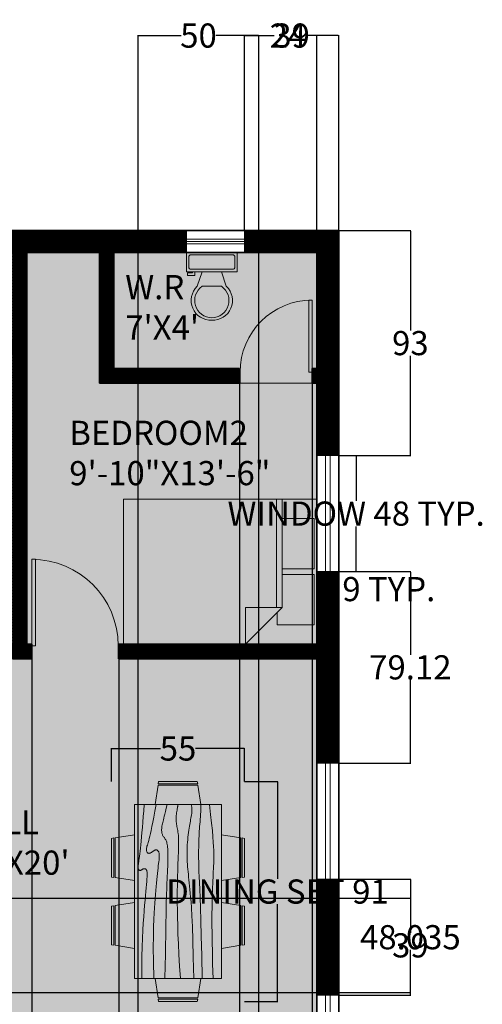
# Model space of a CAD drawing. Units: inches. Extents: x -89252 to 1164, y -183799 to 823.
# Tile 4 of 4: x 972 to 1164, y 416 to 823. Entities that reach past the tile are written whole.
import ezdxf

# ---------------------------------------------------------------- set-up
doc = ezdxf.new("R2010")
doc.units = ezdxf.units.IN
doc.header["$MEASUREMENT"] = 0
for name, color, linetype, lineweight in [('A-ANNO-DIMS', 2, 'Continuous', 18), ('A-AREA-IDEN', 7, 'Continuous', 25), ('A-FURN', 8, 'Continuous', 18), ('A-GLAZ', 4, 'Continuous', 18), ('A-WALL', 7, 'Continuous', 35), ('BED', 7, 'Continuous', 18), ('DOOR', 7, 'Continuous', 18), ('TOILET', 7, 'Continuous', 18)]:
    doc.layers.add(name, color=color, linetype=linetype, lineweight=lineweight)
doc.layers.add('A-FLOR-PATT', color=252, linetype='Continuous', lineweight=13, true_color=0x939598)
doc.layers.add('A-WALL-PATT', color=18, linetype='Continuous', lineweight=13, true_color=0x000000)
doc.styles.get("Standard").update_dxf_attribs({"font": 'arial.ttf'})
doc.dimstyles.get("Standard").update_dxf_attribs({"dimtxt": 10, "dimasz": 0.18, "dimexe": 0.18, "dimexo": 0.0625, "dimgap": 0.09, "dimtad": 0, "dimtih": 1, "dimtoh": 1, "dimdec": 0, "dimzin": 0, "dimdsep": 46, "dimlunit": 3, "dimtxsty": 'Standard', "dimcen": 0.09, "dimadec": 0, "dimazin": 0, "dimtfac": 1, "dimtdec": 0, "dimtofl": 0, "dimtmove": 0, "dimatfit": 3, "dimfxl": 1, "dimtolj": 1, "dimtzin": 0, "dimarcsym": 0})

# ---------------------------------------------------------------- blocks, each defined once
blk = doc.blocks.new('*U3')
for p, q in [((0, 0), (0, -6)), ((40, 0), (40, -6))]:
    blk.add_line(p, q)
blk.add_lwpolyline([(0, 0), (0, 40), (1.75, 40), (1.75, 0)], close=True)
blk.add_arc((0, 0), 40, 0, 90)
blk = doc.blocks.new('Dining Set - 36 x 72 in.')
for p, q in [((-22.2343, 26.00059), (-23.4847, 17.99762)), ((-22.2304, 26), (-5.7608, 26)), ((-22, 27.5), (-22.1562, 26.50042)), ((-5.8416, 26.5), (-22.1534, 26.5)), ((-22, 27.5), (-6, 27.5)), ((-5.8437, 26.49966), (-6, 27.5)), ((-4.5152, 17.99762), (-5.7655, 25.99926)), ((5.7657, 26.00059), (4.5153, 17.99762)), ((5.7696, 26), (22.2392, 26)), ((6, 27.5), (5.8438, 26.50042)), ((22.1584, 26.5), (5.8466, 26.5)), ((6, 27.5), (22, 27.5)), ((22.1563, 26.49966), (22, 27.5)), ((23.4848, 17.99762), (22.2345, 25.99926)), ((36, 18), (-36, 18)), ((-36, 18), (-36, -18)), ((36, -18), (36, 18)), ((-45.5, 8), (-44.5004, 8.15617)), ((-44.5, -8.15843), (-44.5, 8.15338)), ((-44.0006, 8.23428), (-35.9976, 9.48474)), ((-44, 8.23041), (-44, -8.23915)), ((44.0006, 8.23428), (35.9976, 9.48474)), ((44, 8.23041), (44, -8.23915)), ((44.5, -8.15843), (44.5, 8.15338)), ((45.5, 8), (44.5005, 8.15617)), ((-45.5, 8), (-45.5, -8)), ((45.5, 8), (45.5, -8)), ((-44.4997, -8.15631), (-45.5, -8)), ((44.4997, -8.15631), (45.5, -8)), ((-35.9976, -9.48476), (-43.9993, -8.2345)), ((35.9976, -9.48476), (43.9993, -8.2345)), ((-36, -18), (36, -18)), ((-22.2343, -26.0006), (-23.4847, -17.99762)), ((-4.5152, -17.99762), (-5.7655, -25.99928)), ((5.7657, -26.0006), (4.5153, -17.99762)), ((23.4848, -17.99762), (22.2345, -25.99928)), ((-22.2304, -26), (-5.7608, -26)), ((-22, -27.5), (-22.1562, -26.50044)), ((-5.8416, -26.5), (-22.1534, -26.5)), ((-22, -27.5), (-6, -27.5)), ((-5.8437, -26.49967), (-6, -27.5)), ((5.7696, -26), (22.2392, -26)), ((6, -27.5), (5.8438, -26.50044)), ((22.1584, -26.5), (5.8466, -26.5)), ((6, -27.5), (22, -27.5)), ((22.1563, -26.49967), (22, -27.5))]:
    blk.add_line(p, q)
for points in [[(-36, 15), (-31.1772, 14.97754), (-26.8079, 14.91406), (-22.8538, 14.81543), (-19.276, 14.6875), (-16.0362, 14.53613), (-13.0957, 14.36718), (-10.4159, 14.18652), (-7.9583, 14), (-5.6904, 13.81315), (-3.6035, 13.63021), (-1.6954, 13.45508), (0.0365, 13.29166), (1.5945, 13.14388), (2.9811, 13.01562), (4.1988, 12.9108), (5.25, 12.83333), (6.1393, 12.78613), (6.8802, 12.76823), (7.4883, 12.77767), (7.9792, 12.8125), (8.3685, 12.87077), (8.6719, 12.95052), (8.9049, 13.0498), (9.0833, 13.16666), (9.2205, 13.29899), (9.3216, 13.44401), (9.3895, 13.59879), (9.4271, 13.76041), (9.4373, 13.92594), (9.4232, 14.09245), (9.3875, 14.257), (9.3333, 14.41666), (9.2638, 14.56917), (9.1836, 14.71484), (9.0975, 14.85465), (9.0104, 14.98958), (8.9272, 15.1206), (8.8529, 15.2487), (8.7922, 15.37483), (8.75, 15.5), (8.7305, 15.62467), (8.7344, 15.74739), (8.7617, 15.86621), (8.8125, 15.97916), (8.8867, 16.08431), (8.9844, 16.17968), (9.1055, 16.26334), (9.25, 16.33333), (9.4189, 16.38802), (9.6172, 16.42708), (9.8506, 16.45052), (10.125, 16.45833), (10.4463, 16.45052), (10.8203, 16.42708), (11.2529, 16.38802), (11.75, 16.33333), (12.3184, 16.26318), (12.9694, 16.17838), (13.7151, 16.07991), (14.5677, 15.96875), (15.5395, 15.84586), (16.6426, 15.71224), (17.8893, 15.56884), (19.2917, 15.41666), (20.859, 15.25667), (22.5879, 15.08984), (24.4721, 14.91715), (26.5052, 14.73958), (28.6809, 14.5581), (30.9929, 14.3737), (33.4347, 14.18733), (36, 14)], [(-36, 10), (-28.9766, 10.14274), (-23.1725, 10.20442), (-18.4241, 10.19775), (-14.5677, 10.13541), (-11.4399, 10.03011), (-8.877, 9.89453), (-6.7154, 9.74137), (-4.7917, 9.58333), (-2.9698, 9.43082), (-1.2246, 9.28515), (0.4415, 9.14534), (2.026, 9.01041), (3.5266, 8.87939), (4.9408, 8.7513), (6.266, 8.62516), (7.5, 8.5), (8.6411, 8.37549), (9.6914, 8.2539), (10.6538, 8.13818), (11.5312, 8.03125), (12.3267, 7.93603), (13.043, 7.85547), (13.6831, 7.79248), (14.25, 7.75), (14.7471, 7.7303), (15.1797, 7.73307), (15.5537, 7.75732), (15.875, 7.80208), (16.1494, 7.86637), (16.3828, 7.94922), (16.5811, 8.04964), (16.75, 8.16666), (16.8944, 8.29915), (17.0143, 8.44531), (17.1089, 8.60319), (17.1771, 8.77083), (17.218, 8.94629), (17.2305, 9.1276), (17.2137, 9.31282), (17.1667, 9.5), (17.0895, 9.6875), (16.987, 9.875), (16.8649, 10.0625), (16.7292, 10.25), (16.5856, 10.4375), (16.4401, 10.625), (16.2985, 10.8125), (16.1667, 11), (16.05, 11.18733), (15.9518, 11.3737), (15.8752, 11.5581), (15.8229, 11.73958), (15.798, 11.91715), (15.8034, 12.08984), (15.842, 12.25667), (15.9167, 12.41666), (16.0295, 12.56836), (16.1784, 12.70833), (16.3605, 12.83268), (16.5729, 12.9375), (16.8127, 13.01888), (17.0768, 13.07291), (17.3625, 13.0957), (17.6667, 13.08333), (17.9894, 13.03312), (18.3418, 12.94726), (18.7382, 12.82918), (19.1927, 12.68229), (19.7195, 12.51001), (20.3327, 12.31575), (21.0465, 12.10294), (21.875, 11.875), (22.8357, 11.63354), (23.959, 11.37304), (25.2786, 11.08618), (26.8282, 10.76562), (28.6414, 10.40405), (30.752, 9.99414), (33.1936, 9.52856), (36, 9)], [(-36, 5.5), (-30.7157, 5.3348), (-26.069, 5.20963), (-21.9946, 5.11767), (-18.4271, 5.05208), (-15.3009, 5.00602), (-12.5508, 4.97265), (-10.1112, 4.94515), (-7.9167, 4.91666), (-5.909, 4.88167), (-4.0586, 4.83984), (-2.3429, 4.79215), (-0.7396, 4.73958), (0.7739, 4.6831), (2.22, 4.6237), (3.6213, 4.56233), (5, 4.5), (6.373, 4.43782), (7.7344, 4.3776), (9.0723, 4.32129), (10.375, 4.27083), (11.6309, 4.22819), (12.8281, 4.19531), (13.9551, 4.17415), (15, 4.16666), (15.954, 4.17448), (16.819, 4.19791), (17.6001, 4.23698), (18.3021, 4.29166), (18.9299, 4.36198), (19.4883, 4.44791), (19.9823, 4.54948), (20.4167, 4.66666), (20.7969, 4.79899), (21.1302, 4.94401), (21.4245, 5.09879), (21.6875, 5.26041), (21.9271, 5.42594), (22.1511, 5.59245), (22.3672, 5.757), (22.5834, 5.91666), (22.8065, 6.06868), (23.0404, 6.21093), (23.2879, 6.34147), (23.5521, 6.45833), (23.8358, 6.55957), (24.142, 6.64323), (24.4735, 6.70735), (24.8334, 6.75), (25.2235, 6.76969), (25.642, 6.76692), (26.0858, 6.74267), (26.5521, 6.69791), (27.0379, 6.63362), (27.5404, 6.55078), (28.0565, 6.45036), (28.5834, 6.33333), (29.1242, 6.19987), (29.7071, 6.04687), (30.3661, 5.87044), (31.1354, 5.66666), (32.0493, 5.43164), (33.142, 5.16146), (34.4475, 4.85221), (36, 4.5)], [(-36, -1), (-30.7915, -0.6591), (-26.0195, -0.38216), (-21.6519, -0.16284), (-17.6563, 0.00521), (-14.0005, 0.12833), (-10.6523, 0.21289), (-7.5796, 0.26522), (-4.75, 0.29166), (-2.134, 0.29793), (0.2878, 0.28711), (2.5317, 0.26163), (4.6146, 0.22396), (6.5529, 0.17651), (8.3633, 0.12174), (10.0623, 0.06209), (11.6667, 0), (13.1899, -0.06201), (14.6341, -0.1211), (15.9982, -0.17432), (17.2813, -0.21875), (18.4823, -0.25147), (19.6003, -0.26953), (20.6343, -0.27002), (21.5834, -0.25), (22.4481, -0.20768), (23.2357, -0.14584), (23.9549, -0.06836), (24.6146, 0.02083), (25.2235, 0.11784), (25.7904, 0.21875), (26.3241, 0.31966), (26.8334, 0.41666), (27.3265, 0.50618), (27.8099, 0.58593), (28.2894, 0.65397), (28.7709, 0.70833), (29.2601, 0.74707), (29.763, 0.76823), (30.2855, 0.76985), (30.8334, 0.75), (31.4088, 0.70784), (31.9994, 0.64713), (32.589, 0.57275), (33.1615, 0.48958), (33.7008, 0.4025), (34.1908, 0.3164), (34.6153, 0.23616), (34.9584, 0.16666), (35.2099, 0.11165), (35.3848, 0.07031), (35.504, 0.04069), (35.5886, 0.02083), (35.6594, 0.00879), (35.7377, 0.0026), (35.8442, 0.00032), (36, 0)], [(-36, -6.5), (-27.1843, -6.31267), (-20.084, -6.1263), (-14.469, -5.9419), (-10.1094, -5.76042), (-6.7752, -5.58285), (-4.2363, -5.41016), (-2.2629, -5.24333), (-0.625, -5.08334), (0.8708, -4.93099), (2.2715, -4.78646), (3.5872, -4.64974), (4.8281, -4.52084), (6.0046, -4.39974), (7.127, -4.28646), (8.2053, -4.18099), (9.25, -4.08334), (10.2705, -3.99382), (11.2734, -3.91407), (12.2647, -3.84603), (13.25, -3.79167), (14.2354, -3.75293), (15.2266, -3.73177), (16.2295, -3.73015), (17.25, -3.75), (18.2912, -3.79248), (19.3451, -3.85547), (20.4009, -3.93604), (21.4479, -4.03125), (22.4754, -4.13819), (23.4727, -4.25391), (24.4289, -4.37549), (25.3334, -4.5), (26.1785, -4.62492), (26.9694, -4.74935), (27.7145, -4.87281), (28.4219, -4.99479), (29.1, -5.11483), (29.7572, -5.23242), (30.4016, -5.34709), (31.0417, -5.45834), (31.6837, -5.56437), (32.3262, -5.65821), (32.9658, -5.73153), (33.599, -5.77604), (34.2224, -5.78345), (34.8327, -5.74545), (35.4264, -5.65373), (36, -5.5)], [(-36, -10), (-26.4022, -9.81299), (-18.4675, -9.62891), (-11.9839, -9.45069), (-6.7396, -9.28125), (-2.5226, -9.12354), (0.8789, -8.98047), (3.6769, -8.85498), (6.0833, -8.75), (8.2767, -8.66765), (10.3021, -8.60677), (12.1712, -8.56543), (13.8958, -8.54167), (15.4876, -8.53353), (16.9583, -8.53907), (18.3197, -8.55632), (19.5834, -8.58334), (20.7616, -8.61841), (21.8685, -8.66081), (22.9188, -8.71004), (23.9271, -8.76563), (24.9081, -8.82707), (25.8763, -8.89388), (26.8465, -8.96558), (27.8334, -9.04167), (28.8474, -9.12118), (29.8828, -9.20117), (30.93, -9.27824), (31.9792, -9.34896), (33.0205, -9.40991), (34.0443, -9.45768), (35.0407, -9.48885), (36, -9.5)], [(-36, -14.5), (-30.0881, -14.33513), (-25.0332, -14.21224), (-20.7312, -14.12647), (-17.0781, -14.07292), (-13.97, -14.04671), (-11.3027, -14.04297), (-8.9724, -14.05681), (-6.875, -14.08334), (-4.9224, -14.11833), (-3.0905, -14.16016), (-1.3709, -14.20785), (0.2448, -14.26042), (1.7647, -14.3169), (3.1973, -14.3763), (4.5507, -14.43767), (5.8333, -14.5), (7.0554, -14.5621), (8.235, -14.62175), (9.3922, -14.67652), (10.5469, -14.72396), (11.7192, -14.76164), (12.929, -14.78711), (14.1965, -14.79794), (15.5417, -14.79167), (16.9933, -14.76424), (18.6152, -14.70508), (20.4804, -14.60197), (22.6615, -14.44271), (25.2312, -14.21509), (28.2624, -13.9069), (31.8277, -13.50594), (36, -13)]]:
    blk.add_lwpolyline(points)
blk = doc.blocks.new('Bed - Queen')
for p, q in [((0, -80.00003), (0, 0)), ((0, 0), (59.99999, 0)), ((59.99999, 0), (59.99999, -80.00003)), ((7.99999, -1.2), (28.79998, -1.2)), ((7.99999, -14.4), (7.99999, -1.2)), ((28.79998, -1.2), (28.79998, -14.4)), ((31.19999, -1.2), (51.99999, -1.2)), ((31.19999, -14.4), (31.19999, -1.2)), ((51.99999, -1.2), (51.99999, -16.4)), ((0, -14.4), (44.8, -14.4)), ((59.99999, -29.6), (44.8, -14.4)), ((44.8, -14.4), (44.8, -29.6)), ((44.8, -16.8), (0, -16.8)), ((51.99999, -16.4), (46.79936, -16.4)), ((44.8, -29.6), (59.99999, -29.6)), ((59.99999, -80.00003), (0, -80.00003))]:
    blk.add_line(p, q)
blk = doc.blocks.new('*U12')
for p, q in [((9.5, -6), (9.5, -2)), ((-8, -8.5), (-8, -8)), ((-7, -8), (-7, -9.5)), ((-4, -8), (-6, -14)), ((4, -8), (6, -14)), ((-10, -8.5), (-8, -8.5)), ((-10, -9.5), (-10, -8.5)), ((-7, -9.5), (-10, -9.5)), ((4, -14), (-4, -14))]:
    blk.add_line(p, q)
blk.add_lwpolyline([(10.5, -8), (10.5, 0), (-10.5, 0), (-10.5, -8)], close=True)
for points in [[(-9.5, -2), (-9.5, -6)], [(8.5, -1), (-8.5, -1)], [(-8.5, -7), (8.5, -7)]]:
    blk.add_lwpolyline(points)
for centre, radius, start, end in [((-8.625, -1.875), 0.8839, 81.8699, 188.1301), ((8.625, -1.875), 0.8839, 351.8699, 98.1301), ((-8.625, -6.125), 0.8839, 171.869898, 278.1301), ((8.625, -6.125), 0.8839, 261.8699, 8.1301), ((-0.4772, -19.9188), 8.0953, 133.01722, 273.38), ((0.0374, -19.8731), 7.127, 124.50543, 269.7), ((-0.0373, -19.8731), 7.127, 270.3, 55.4946), ((0.4773, -19.9188), 8.0953, 266.62, 46.9828)]:
    blk.add_arc(centre, radius, start, end)
blk = doc.blocks.new('WIN-24IN-9IN-WALL')
for p, q in [((9, 24), (0, 24)), ((3.5, 0), (3.5, 24)), ((4.5, 0), (4.5, 24)), ((5.5, 0), (5.5, 24)), ((9, 0), (0, 0))]:
    blk.add_line(p, q)
blk = doc.blocks.new('WIN-48IN-9IN-WALL')
for p, q in [((0, 48), (9, 48)), ((3.5, 0), (3.5, 48)), ((5.5, 0), (5.5, 48)), ((0, 0), (9, 0))]:
    blk.add_line(p, q)
blk = doc.blocks.new('*D24')
at = {"layer": 'A-ANNO-DIMS', "color": 0, "lineweight": -2, "transparency": 16777216}
for p, q in [((1104.43, 642.39), (1111.74, 642.39)), ((1111.56, 642.21), (1111.56, 623.65)), ((1111.56, 594.57), (1111.56, 613.13)), ((1104.43, 594.39), (1111.74, 594.39))]:
    blk.add_line(p, q, dxfattribs=at)
at = {"layer": 'A-ANNO-DIMS', "color": 0, "transparency": 16777216}
for points in [[(1111.53, 642.21), (1111.59, 642.21), (1111.56, 642.39)], [(1111.53, 594.57), (1111.59, 594.57), (1111.56, 594.39)]]:
    blk.add_solid(points, dxfattribs=at)
at = {"layer": 'Defpoints', "color": 0, "transparency": 16777216}
for p in [(1104.36, 642.39), (1111.56, 642.39), (1104.36, 594.39)]:
    blk.add_point(p, dxfattribs=at)
at = {"layer": 'A-ANNO-DIMS', "color": 0, "transparency": 16777216, "insert": (1111.56, 618.39), "char_height": 10, "attachment_point": 5}
blk.add_mtext('\\A1;WINDOW 48 TYP.', dxfattribs=at)
blk = doc.blocks.new('*D25')
at = {"layer": 'A-ANNO-DIMS', "color": 0, "lineweight": -2, "transparency": 16777216}
for p, q in [((1095.36, 594.33), (1095.36, 587.01)), ((1104.36, 594.33), (1104.36, 587.01)), ((1095.54, 587.19), (1104.18, 587.19)), ((1104.36, 587.19), (1104.54, 587.19))]:
    blk.add_line(p, q, dxfattribs=at)
at = {"layer": 'A-ANNO-DIMS', "color": 0, "transparency": 16777216}
for points in [[(1095.54, 587.22), (1095.54, 587.16), (1095.36, 587.19)], [(1104.18, 587.22), (1104.18, 587.16), (1104.36, 587.19)]]:
    blk.add_solid(points, dxfattribs=at)
at = {"layer": 'Defpoints', "color": 0, "transparency": 16777216}
for p in [(1095.36, 594.39), (1104.36, 594.39), (1104.36, 587.19)]:
    blk.add_point(p, dxfattribs=at)
at = {"layer": 'A-ANNO-DIMS', "color": 0, "transparency": 16777216, "insert": (1125.09, 587.19), "char_height": 10, "attachment_point": 5}
blk.add_mtext('\\A1;9 TYP.', dxfattribs=at)
blk = doc.blocks.new('*D28')
at = {"layer": 'A-ANNO-DIMS', "color": 0, "lineweight": -2, "transparency": 16777216}
for p, q in [((1065.43, 507.63), (1079.2, 507.63)), ((1079.02, 507.45), (1079.02, 467.39)), ((1079.02, 416.81), (1079.02, 456.87)), ((1065.43, 416.63), (1079.2, 416.63))]:
    blk.add_line(p, q, dxfattribs=at)
at = {"layer": 'A-ANNO-DIMS', "color": 0, "transparency": 16777216}
for points in [[(1078.99, 507.45), (1079.05, 507.45), (1079.02, 507.63)], [(1078.99, 416.81), (1079.05, 416.81), (1079.02, 416.63)]]:
    blk.add_solid(points, dxfattribs=at)
at = {"layer": 'Defpoints', "color": 0, "transparency": 16777216}
for p in [(1065.37, 507.63), (1079.02, 507.63), (1065.37, 416.63)]:
    blk.add_point(p, dxfattribs=at)
at = {"layer": 'A-ANNO-DIMS', "color": 0, "transparency": 16777216, "insert": (1079.02, 462.13), "char_height": 10, "attachment_point": 5}
blk.add_mtext('\\A1;DINING SET 91', dxfattribs=at)
blk = doc.blocks.new('*D29')
at = {"layer": 'A-ANNO-DIMS', "color": 0, "lineweight": -2, "transparency": 16777216}
for p, q in [((1010.37, 507.7), (1010.37, 521.46)), ((1010.55, 521.28), (1030.58, 521.28)), ((1065.19, 521.28), (1045.16, 521.28)), ((1065.37, 507.7), (1065.37, 521.46))]:
    blk.add_line(p, q, dxfattribs=at)
at = {"layer": 'A-ANNO-DIMS', "color": 0, "transparency": 16777216}
for points in [[(1010.55, 521.31), (1010.55, 521.25), (1010.37, 521.28)], [(1065.19, 521.31), (1065.19, 521.25), (1065.37, 521.28)]]:
    blk.add_solid(points, dxfattribs=at)
at = {"layer": 'Defpoints', "color": 0, "transparency": 16777216}
for p in [(1010.37, 521.28), (1010.37, 507.63), (1065.37, 507.63)]:
    blk.add_point(p, dxfattribs=at)
at = {"layer": 'A-ANNO-DIMS', "color": 0, "transparency": 16777216, "insert": (1037.87, 521.28), "char_height": 10, "attachment_point": 5}
blk.add_mtext('\\A1;55', dxfattribs=at)
blk = doc.blocks.new('*D34')
at = {"layer": 'A-ANNO-DIMS', "color": 0, "lineweight": -2, "transparency": 16777216}
for p, q in [((1021.36, 318.45), (1021.36, 816.22)), ((1021.54, 816.04), (1039.13, 816.04)), ((1071.18, 816.04), (1053.6, 816.04)), ((1071.36, 318.45), (1071.36, 816.22))]:
    blk.add_line(p, q, dxfattribs=at)
at = {"layer": 'A-ANNO-DIMS', "color": 0, "transparency": 16777216}
for points in [[(1021.54, 816.07), (1021.54, 816.01), (1021.36, 816.04)], [(1071.18, 816.07), (1071.18, 816.01), (1071.36, 816.04)]]:
    blk.add_solid(points, dxfattribs=at)
at = {"layer": 'Defpoints', "color": 0, "transparency": 16777216}
for p in [(1071.36, 816.04), (1021.36, 318.39), (1071.36, 318.39)]:
    blk.add_point(p, dxfattribs=at)
at = {"layer": 'A-ANNO-DIMS', "color": 0, "transparency": 16777216, "insert": (1046.36, 816.04), "char_height": 10, "attachment_point": 5}
blk.add_mtext('\\A1;50', dxfattribs=at)
blk = doc.blocks.new('*D35')
at = {"layer": 'A-ANNO-DIMS', "color": 0, "lineweight": -2, "transparency": 16777216}
for p, q in [((1104.43, 735.39), (1134.19, 735.39)), ((1134.01, 735.21), (1134.01, 694.09)), ((1134.01, 642.57), (1134.01, 683.69)), ((1104.43, 642.39), (1134.19, 642.39))]:
    blk.add_line(p, q, dxfattribs=at)
at = {"layer": 'A-ANNO-DIMS', "color": 0, "transparency": 16777216}
for points in [[(1133.98, 735.21), (1134.04, 735.21), (1134.01, 735.39)], [(1133.98, 642.57), (1134.04, 642.57), (1134.01, 642.39)]]:
    blk.add_solid(points, dxfattribs=at)
at = {"layer": 'Defpoints', "color": 0, "transparency": 16777216}
for p in [(1104.36, 735.39), (1134.01, 735.39), (1104.36, 642.39)]:
    blk.add_point(p, dxfattribs=at)
at = {"layer": 'A-ANNO-DIMS', "color": 0, "transparency": 16777216, "insert": (1134.01, 688.89), "char_height": 10, "attachment_point": 5}
blk.add_mtext('\\A1;93', dxfattribs=at)
blk = doc.blocks.new('*D36')
at = {"layer": 'A-ANNO-DIMS', "color": 0, "lineweight": -2, "transparency": 16777216}
for p, q in [((1104.43, 594.39), (1134.19, 594.39)), ((1134.01, 594.21), (1134.01, 560.03)), ((1134.01, 515.45), (1134.01, 549.63)), ((1104.43, 515.27), (1134.19, 515.27))]:
    blk.add_line(p, q, dxfattribs=at)
at = {"layer": 'A-ANNO-DIMS', "color": 0, "transparency": 16777216}
for points in [[(1133.98, 594.21), (1134.04, 594.21), (1134.01, 594.39)], [(1133.98, 515.45), (1134.04, 515.45), (1134.01, 515.27)]]:
    blk.add_solid(points, dxfattribs=at)
at = {"layer": 'Defpoints', "color": 0, "transparency": 16777216}
for p in [(1104.36, 594.39), (1104.36, 515.27), (1134.01, 515.27)]:
    blk.add_point(p, dxfattribs=at)
at = {"layer": 'A-ANNO-DIMS', "color": 0, "transparency": 16777216, "insert": (1134.01, 554.83), "char_height": 10, "attachment_point": 5}
blk.add_mtext('\\A1;79.12', dxfattribs=at)
blk = doc.blocks.new('*D37')
at = {"layer": 'A-ANNO-DIMS', "color": 0, "lineweight": -2, "transparency": 16777216}
for p, q in [((1104.43, 467.27), (1134.19, 467.27)), ((1134.01, 467.09), (1134.01, 448.45)), ((1134.01, 419.41), (1134.01, 438.05)), ((1104.43, 419.23), (1134.19, 419.23))]:
    blk.add_line(p, q, dxfattribs=at)
at = {"layer": 'A-ANNO-DIMS', "color": 0, "transparency": 16777216}
for points in [[(1133.98, 467.09), (1134.04, 467.09), (1134.01, 467.27)], [(1133.98, 419.41), (1134.04, 419.41), (1134.01, 419.23)]]:
    blk.add_solid(points, dxfattribs=at)
at = {"layer": 'Defpoints', "color": 0, "transparency": 16777216}
for p in [(1104.36, 467.27), (1104.36, 419.23), (1134.01, 419.23)]:
    blk.add_point(p, dxfattribs=at)
at = {"layer": 'A-ANNO-DIMS', "color": 0, "transparency": 16777216, "insert": (1134.01, 443.25), "char_height": 10, "attachment_point": 5}
blk.add_mtext('\\A1;48.035', dxfattribs=at)
blk = doc.blocks.new('*D39')
at = {"layer": 'A-ANNO-DIMS', "color": 0, "lineweight": -2, "transparency": 16777216}
for p, q in [((977.36, 564.33), (977.36, 165.56)), ((1013.36, 564.33), (1013.36, 165.56)), ((977.54, 165.74), (988.12, 165.74)), ((1013.18, 165.74), (1002.61, 165.74))]:
    blk.add_line(p, q, dxfattribs=at)
at = {"layer": 'A-ANNO-DIMS', "color": 0, "transparency": 16777216}
for points in [[(977.54, 165.77), (977.54, 165.71), (977.36, 165.74)], [(1013.18, 165.77), (1013.18, 165.71), (1013.36, 165.74)]]:
    blk.add_solid(points, dxfattribs=at)
at = {"layer": 'Defpoints', "color": 0, "transparency": 16777216}
for p in [(977.36, 564.39), (1013.36, 564.39), (1013.36, 165.74)]:
    blk.add_point(p, dxfattribs=at)
at = {"layer": 'A-ANNO-DIMS', "color": 0, "transparency": 16777216, "insert": (995.36, 165.74), "char_height": 10, "attachment_point": 5}
blk.add_mtext('\\A1;36', dxfattribs=at)
blk = doc.blocks.new('*D40')
at = {"layer": 'A-ANNO-DIMS', "color": 0, "lineweight": -2, "transparency": 16777216}
for p, q in [((1063.36, 672.33), (1063.36, 165.56)), ((1093.36, 672.33), (1093.36, 165.56)), ((1063.54, 165.74), (1071.13, 165.74)), ((1093.18, 165.74), (1085.6, 165.74))]:
    blk.add_line(p, q, dxfattribs=at)
at = {"layer": 'A-ANNO-DIMS', "color": 0, "transparency": 16777216}
for points in [[(1063.54, 165.77), (1063.54, 165.71), (1063.36, 165.74)], [(1093.18, 165.77), (1093.18, 165.71), (1093.36, 165.74)]]:
    blk.add_solid(points, dxfattribs=at)
at = {"layer": 'Defpoints', "color": 0, "transparency": 16777216}
for p in [(1063.36, 672.39), (1093.36, 672.39), (1093.36, 165.74)]:
    blk.add_point(p, dxfattribs=at)
at = {"layer": 'A-ANNO-DIMS', "color": 0, "transparency": 16777216, "insert": (1078.36, 165.74), "char_height": 10, "attachment_point": 5}
blk.add_mtext('\\A1;30', dxfattribs=at)
blk = doc.blocks.new('*D42')
at = {"layer": 'A-ANNO-DIMS', "color": 0, "lineweight": -2, "transparency": 16777216}
for p, q in [((1065.36, 735.45), (1065.36, 816.22)), ((1065.54, 816.04), (1077.6, 816.04)), ((1104.18, 816.04), (1092.12, 816.04)), ((1104.36, 735.45), (1104.36, 816.22))]:
    blk.add_line(p, q, dxfattribs=at)
at = {"layer": 'A-ANNO-DIMS', "color": 0, "transparency": 16777216}
for points in [[(1065.54, 816.07), (1065.54, 816.01), (1065.36, 816.04)], [(1104.18, 816.07), (1104.18, 816.01), (1104.36, 816.04)]]:
    blk.add_solid(points, dxfattribs=at)
at = {"layer": 'Defpoints', "color": 0, "transparency": 16777216}
for p in [(1065.36, 816.04), (1065.36, 735.39), (1104.36, 735.39)]:
    blk.add_point(p, dxfattribs=at)
at = {"layer": 'A-ANNO-DIMS', "color": 0, "transparency": 16777216, "insert": (1084.86, 816.04), "char_height": 10, "attachment_point": 5}
blk.add_mtext('\\A1;39', dxfattribs=at)
blk = doc.blocks.new('*D46')
at = {"layer": 'A-ANNO-DIMS', "color": 0, "lineweight": -2, "transparency": 16777216}
for p, q in [((1071.36, 318.45), (1071.36, 816.22)), ((1071.54, 816.04), (1076.05, 816.04)), ((1095.18, 816.04), (1090.68, 816.04)), ((1095.36, 318.45), (1095.36, 816.22))]:
    blk.add_line(p, q, dxfattribs=at)
at = {"layer": 'A-ANNO-DIMS', "color": 0, "transparency": 16777216}
for points in [[(1071.54, 816.07), (1071.54, 816.01), (1071.36, 816.04)], [(1095.18, 816.07), (1095.18, 816.01), (1095.36, 816.04)]]:
    blk.add_solid(points, dxfattribs=at)
at = {"layer": 'Defpoints', "color": 0, "transparency": 16777216}
for p in [(1095.36, 816.04), (1071.36, 318.39), (1095.36, 318.39)]:
    blk.add_point(p, dxfattribs=at)
at = {"layer": 'A-ANNO-DIMS', "color": 0, "transparency": 16777216, "insert": (1083.36, 816.04), "char_height": 10, "attachment_point": 5}
blk.add_mtext('\\A1;24', dxfattribs=at)
blk = doc.blocks.new('*D52')
at = {"layer": 'A-ANNO-DIMS', "color": 0, "lineweight": -2, "transparency": 16777216}
for p, q in [((859.43, 459.39), (1134.19, 459.39)), ((1134.01, 459.21), (1134.01, 445.09)), ((1134.01, 420.57), (1134.01, 434.69)), ((859.43, 420.39), (1134.19, 420.39))]:
    blk.add_line(p, q, dxfattribs=at)
at = {"layer": 'A-ANNO-DIMS', "color": 0, "transparency": 16777216}
for points in [[(1133.98, 459.21), (1134.04, 459.21), (1134.01, 459.39)], [(1133.98, 420.57), (1134.04, 420.57), (1134.01, 420.39)]]:
    blk.add_solid(points, dxfattribs=at)
at = {"layer": 'Defpoints', "color": 0, "transparency": 16777216}
for p in [(859.36, 459.39), (1134.01, 459.39), (859.36, 420.39)]:
    blk.add_point(p, dxfattribs=at)
at = {"layer": 'A-ANNO-DIMS', "color": 0, "transparency": 16777216, "insert": (1134.01, 439.89), "char_height": 10, "attachment_point": 5}
blk.add_mtext('\\A1;39', dxfattribs=at)

msp = doc.modelspace()

# ---------------------------------------------------------------- hatches: boundary and pattern name
at = {"layer": 'A-FLOR-PATT'}
h = msp.add_hatch(color=256, dxfattribs=at)
h.dxf.hatch_style = 1
h.paths.add_polyline_path([(1095.364, 558.3893), (1013.364, 558.3893), (1013.364, 564.3893), (1095.364, 564.3893), (1095.364, 672.3893), (1093.364, 672.3893), (1063.364, 672.3893), (1005.364, 672.3893), (1005.364, 726.3893), (975.364, 726.3893), (975.364, 690.3893), (975.364, 564.3893), (977.364, 564.3893), (977.364, 558.3893), (975.364, 558.3893), (969.364, 558.3893), (967.364, 558.3893), (967.364, 564.3893), (969.364, 564.3893), (969.364, 684.3893), (967.364, 684.3893), (937.364, 684.3893), (891.364, 684.3893), (891.364, 588.3893), (929.3053, 588.3893), (929.3053, 564.3893), (937.364, 564.3893), (937.364, 558.3893), (857.364, 558.3893), (857.364, 564.3893), (861.364, 564.3893), (861.364, 684.3893), (729.364, 684.3893), (729.364, 564.3893), (781.364, 564.3893), (781.364, 558.3893), (729.364, 558.3893), (729.364, 510.3893), (813.364, 510.3893), (813.364, 558.3893), (811.364, 558.3893), (811.364, 564.3893), (813.364, 564.3893), (819.364, 564.3893), (821.364, 564.3893), (821.364, 558.3893), (819.364, 558.3893), (819.364, 510.3893), (859.364, 510.3893), (859.364, 420.3893), (903.364, 420.3893), (903.364, 414.3893), (903.364, 412.3893), (897.364, 412.3893), (897.364, 414.3893), (813.364, 414.3893), (813.364, 366.3893), (897.364, 366.3893), (897.364, 382.3893), (903.364, 382.3893), (903.364, 360.3893), (903.364, 358.3893), (897.364, 358.3893), (897.364, 360.3893), (807.364, 360.3893), (805.364, 360.3893), (805.364, 366.3893), (807.364, 366.3893), (807.364, 414.3893), (729.364, 414.3893), (729.364, 366.3893), (775.364, 366.3893), (775.364, 360.3893), (729.364, 360.3893), (729.364, 240.3893), (897.364, 240.3893), (897.364, 318.3893), (1021.364, 318.3893), (1021.364, 312.3893), (1071.364, 312.3893), (1071.364, 318.3893), (1095.364, 318.3893)])
h.paths.add_polyline_path([(1095.364, 726.3893), (1011.364, 726.3893), (1011.364, 678.3893), (1063.364, 678.3893), (1063.364, 672.3893), (1093.364, 672.3893), (1093.364, 678.3893), (1095.364, 678.3893)])
h.paths.add_polyline_path([(969.364, 726.3893), (729.364, 726.3893), (729.364, 690.3893), (937.364, 690.3893), (937.364, 684.3893), (967.364, 684.3893), (967.364, 690.3893), (969.364, 690.3893)])
at = {"layer": 'A-WALL-PATT'}
h = msp.add_hatch(dxfattribs=at)
h.set_pattern_fill('ANSI31', color=256)
h.paths.add_polyline_path([(867.364, 684.3893), (878.364, 684.3893), (878.364, 690.3893), (817.6735, 690.3893), (817.6735, 684.3893), (861.364, 684.3893), (861.364, 564.3893), (857.364, 564.3893), (857.364, 558.3893), (937.364, 558.3893), (937.364, 564.3893), (867.364, 564.3893)], flags=17)
h.paths.add_polyline_path([(1041.364, 735.3893), (720.364, 735.3893), (720.364, 546.3893), (729.364, 546.3893), (729.364, 558.3893), (781.364, 558.3893), (781.364, 564.3893), (729.364, 564.3893), (729.364, 684.3893), (769.6735, 684.3893), (769.6735, 690.3893), (729.364, 690.3893), (729.364, 726.3893), (969.364, 726.3893), (969.364, 690.3893), (967.364, 690.3893), (967.364, 684.3893), (969.364, 684.3893), (969.364, 564.3893), (967.364, 564.3893), (967.364, 558.3893), (969.364, 558.3893), (975.364, 558.3893), (977.364, 558.3893), (977.364, 564.3893), (975.364, 564.3893), (975.364, 690.3893), (975.364, 726.3893), (1005.364, 726.3893), (1005.364, 672.3893), (1063.364, 672.3893), (1063.364, 678.3893), (1011.364, 678.3893), (1011.364, 726.3893), (1041.364, 726.3893)])
h.paths.add_polyline_path([(1104.364, 735.3893), (1065.364, 735.3893), (1065.364, 726.3893), (1095.364, 726.3893), (1095.364, 678.3893), (1093.364, 678.3893), (1093.364, 672.3893), (1095.364, 672.3893), (1095.364, 642.3893), (1104.364, 642.3893)])
h.paths.add_polyline_path([(1104.364, 594.3893), (1095.364, 594.3893), (1095.364, 564.3893), (1013.364, 564.3893), (1013.364, 558.3893), (1095.364, 558.3893), (1095.364, 515.2697), (1104.364, 515.2697)])
h.paths.add_polyline_path([(1104.364, 467.2697), (1095.364, 467.2697), (1095.364, 419.2348), (1104.364, 419.2348)])
h.paths.add_polyline_path([(1104.364, 371.2348), (1095.364, 371.2348), (1095.364, 312.3893), (1104.364, 312.3893)], flags=17)
h.paths.add_polyline_path([(1095.364, 318.3893), (1071.364, 318.3893), (1071.364, 312.3893), (1095.364, 312.3893)], flags=17)
h.paths.add_polyline_path([(1021.364, 318.3893), (897.364, 318.3893), (897.364, 240.3893), (837.364, 240.3893), (837.364, 234.3893), (903.364, 234.3893), (903.364, 312.3893), (1021.364, 312.3893)], flags=17)
h.paths.add_polyline_path([(903.364, 382.3893), (897.364, 382.3893), (897.364, 366.3893), (813.364, 366.3893), (813.364, 414.3893), (897.364, 414.3893), (897.364, 412.3893), (903.364, 412.3893), (903.364, 414.3893), (903.364, 420.3893), (729.364, 420.3893), (729.364, 504.3893), (859.364, 504.3893), (859.364, 510.3893), (819.364, 510.3893), (819.364, 558.3893), (821.364, 558.3893), (821.364, 564.3893), (819.364, 564.3893), (813.364, 564.3893), (811.364, 564.3893), (811.364, 558.3893), (813.364, 558.3893), (813.364, 510.3893), (729.364, 510.3893), (729.364, 522.3893), (720.364, 522.3893), (720.364, 400.5349), (729.364, 400.5349), (729.364, 414.3893), (807.364, 414.3893), (807.364, 366.3893), (805.364, 366.3893), (805.364, 360.3893), (807.364, 360.3893), (897.364, 360.3893), (897.364, 358.3893), (903.364, 358.3893), (903.364, 360.3893)])
h.paths.add_polyline_path([(775.364, 366.3893), (729.364, 366.3893), (729.364, 376.5349), (720.364, 376.5349), (720.364, 195.3893), (1104.364, 195.3893), (1104.364, 204.3893), (729.364, 204.3893), (729.364, 234.3893), (789.364, 234.3893), (789.364, 240.3893), (729.364, 240.3893), (729.364, 360.3893), (775.364, 360.3893)])
h.paths.add_polyline_path([(937.364, 690.3893), (926.364, 690.3893), (926.364, 684.3893), (937.364, 684.3893)], flags=17)

# ---------------------------------------------------------------- linework, layer by layer
at = {"layer": 'A-WALL'}
for p, q in [((1104.364, 735.3893), (720.364, 735.3893)), ((1104.364, 312.3893), (1104.364, 735.3893)), ((975.364, 690.3893), (975.364, 726.3893)), ((1005.364, 726.3893), (975.364, 726.3893)), ((1005.364, 672.3893), (1005.364, 726.3893)), ((1095.364, 726.3893), (1011.364, 726.3893)), ((1011.364, 678.3893), (1011.364, 726.3893)), ((1011.364, 726.3893), (1095.364, 726.3893)), ((1095.364, 678.3893), (1095.364, 726.3893)), ((975.364, 564.3893), (975.364, 690.3893)), ((1063.364, 678.3893), (1011.364, 678.3893)), ((1063.364, 672.3893), (1063.364, 678.3893)), ((1095.364, 678.3893), (1093.364, 678.3893)), ((1093.364, 678.3893), (1093.364, 672.3893)), ((1063.364, 672.3893), (1005.364, 672.3893)), ((1093.364, 672.3893), (1095.364, 672.3893)), ((1095.364, 564.3893), (1095.364, 672.3893)), ((1095.364, 564.3893), (1095.364, 672.3893)), ((977.364, 564.3893), (975.364, 564.3893)), ((977.364, 558.3893), (977.364, 564.3893)), ((1095.364, 564.3893), (1013.364, 564.3893)), ((1013.364, 558.3893), (1013.364, 564.3893)), ((975.364, 558.3893), (969.364, 558.3893)), ((975.364, 558.3893), (977.364, 558.3893)), ((1095.364, 558.3893), (1013.364, 558.3893)), ((1095.364, 312.3893), (1095.364, 558.3893))]:
    msp.add_line(p, q, dxfattribs=at)
at = {"layer": 'DOOR'}
msp.add_line((1063.364, 672.3893), (1093.364, 672.3893), dxfattribs=at)

# ---------------------------------------------------------------- block references
at = {"layer": 'A-FURN', "rotation": 90}
msp.add_blockref('Dining Set - 36 x 72 in.', (1037.8659, 462.1336), dxfattribs=at)
at = {"layer": 'A-GLAZ'}
for name, p, rotation in [('WIN-24IN-9IN-WALL', (1041.3637, 735.3894), 269.9999999999999), ('WIN-48IN-9IN-WALL', (1104.3641, 515.27), 180), ('WIN-48IN-9IN-WALL', (1104.3641, 419.2351), 180)]:
    msp.add_blockref(name, p, dxfattribs=dict(at, rotation=rotation))
msp.add_blockref('WIN-48IN-9IN-WALL', (1095.364, 594.389), dxfattribs=at)
at = {"layer": 'BED', "rotation": 270}
msp.add_blockref('Bed - Queen', (1095.364, 624.3893), dxfattribs=at)
at = {"layer": 'DOOR'}
for p, xscale, yscale, zscale in [((1093.364, 676.863), -0.7456098286251903, 0.7456098286251903, 0.7456098286251903), ((977.364, 563.7517), 0.8937210586509982, 0.8937210586509982, 0.8937210586509982)]:
    msp.add_blockref('*U3', p, dxfattribs=dict(at, xscale=xscale, yscale=yscale, zscale=zscale))
at = {"layer": 'TOILET'}
msp.add_blockref('*U12', (1051.864, 726.3893), dxfattribs=at)

# ---------------------------------------------------------------- texts
at = {"layer": 'A-AREA-IDEN', "char_height": 10, "attachment_point": 1}
for s, insert in [("W.R\\P7'X4'", (1016.0323, 717.0234)), ('BEDROOM2\\P9\'-10"X13\'-6"', (992.8674, 656.7909)), ("HALL\\P16'X20'", (947.3283, 495.7486))]:
    msp.add_mtext_dynamic_manual_height_columns(s, width=99.889598, gutter_width=1, heights=[0], dxfattribs=dict(at, insert=insert))

# ---------------------------------------------------------------- dimensions: what is measured, and where the dimension line sits
at = {"layer": 'A-ANNO-DIMS'}
for base, p1, p2, picture, middle in [((1071.364, 816.0393), (1021.364, 318.3893), (1071.364, 318.3893), '*D34', (1046.364, 816.0393)), ((1065.364, 816.0393), (1104.364, 735.3893), (1065.364, 735.3893), '*D42', (1084.864, 816.0393)), ((1095.364, 816.0393), (1071.364, 318.3893), (1095.364, 318.3893), '*D46', (1083.364, 816.0393)), ((1093.364, 165.7393), (1063.364, 672.3893), (1093.364, 672.3893), '*D40', (1078.364, 165.7393)), ((1013.364, 165.7393), (977.364, 564.3893), (1013.364, 564.3893), '*D39', (995.364, 165.7393))]:
    dim = msp.add_linear_dim(base=base, p1=p1, p2=p2, dimstyle='Standard', override={"dimdec": 0, "dimlfac": 1, "dimrnd": 0, "dimzin": 0, "dimdsep": 46, "dimlunit": 2}, dxfattribs=at)
    dim.commit()
    dim.dimension.update_dxf_attribs({"geometry": picture, "text_midpoint": middle})
for base, p1, p2, angle, override, picture, middle in [((1134.014, 735.3893), (1104.364, 642.3893), (1104.364, 735.3893), 90, {"dimdec": 0, "dimlfac": 1, "dimrnd": 0, "dimzin": 0, "dimdsep": 46, "dimlunit": 2}, '*D35', (1134.014, 688.8893)), ((1134.014, 515.2697), (1104.364, 594.3893), (1104.364, 515.2697), 90, {"dimdec": 2, "dimlfac": 1, "dimrnd": 0, "dimzin": 0, "dimdsep": 46, "dimlunit": 2}, '*D36', (1134.014, 554.8295)), ((1010.3659, 521.2836), (1065.3659, 507.6336), (1010.3659, 507.6336), 180, {"dimdec": 0, "dimlfac": 1, "dimrnd": 0, "dimzin": 0, "dimdsep": 46, "dimlunit": 2}, '*D29', (1037.8659, 521.2836)), ((1134.014, 419.2348), (1104.364, 467.2697), (1104.364, 419.2348), 90, {"dimdec": 3, "dimlfac": 1, "dimrnd": 0, "dimzin": 0, "dimdsep": 46, "dimlunit": 2}, '*D37', (1134.014, 443.2522)), ((1134.014, 459.3893), (859.364, 420.3893), (859.364, 459.3893), 90, {"dimdec": 0, "dimlfac": 1, "dimrnd": 0, "dimzin": 0, "dimdsep": 46, "dimlunit": 2}, '*D52', (1134.014, 439.8893))]:
    dim = msp.add_linear_dim(base=base, p1=p1, p2=p2, angle=angle, dimstyle='Standard', override=override, dxfattribs=at)
    dim.commit()
    dim.dimension.update_dxf_attribs({"geometry": picture, "text_midpoint": middle})
for base, p1, p2, text, picture, middle in [((1111.564, 642.3893), (1104.364, 594.3893), (1104.364, 642.3893), 'WINDOW <> TYP.', '*D24', (1111.564, 618.3893)), ((1079.0159, 507.6336), (1065.3659, 416.6336), (1065.3659, 507.6336), 'DINING SET <>', '*D28', (1079.0159, 462.1336))]:
    dim = msp.add_linear_dim(base=base, p1=p1, p2=p2, angle=90, text=text, dimstyle='Standard', override={"dimdec": 0, "dimlfac": 1, "dimrnd": 0, "dimzin": 0, "dimdsep": 46, "dimlunit": 2}, dxfattribs=at)
    dim.commit()
    dim.dimension.update_dxf_attribs({"geometry": picture, "text_midpoint": middle})
dim = msp.add_linear_dim(base=(1104.364, 587.1893), p1=(1095.364, 594.3893), p2=(1104.364, 594.3893), text='<> TYP.', dimstyle='Standard', override={"dimdec": 0, "dimlfac": 1, "dimrnd": 0, "dimzin": 0, "dimdsep": 46, "dimlunit": 2}, dxfattribs=at)
dim.commit()
dim.dimension.update_dxf_attribs({"geometry": '*D25', "text_midpoint": (1125.0876, 587.1893)})

doc.saveas('drawing.dxf')
